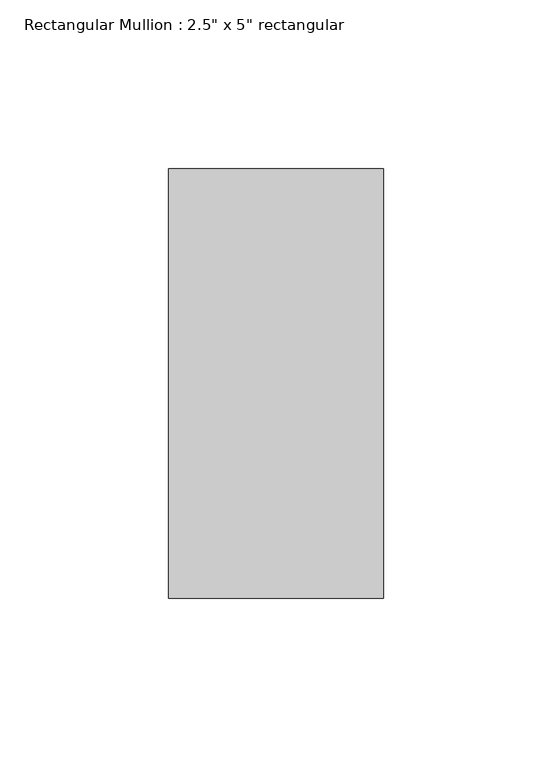
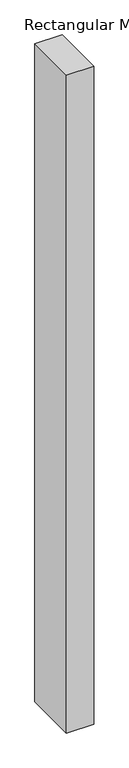
"""IFC4 building model written with IfcOpenShell, lengths in millimetres: member geometry."""

from ifc_helpers import new_model, si_unit, frame, origin, place, context, project, spatial, polyline, outline, extrude, source, transform, mapped, element, save


def member_25f01624(model_context):
    return source(origin(), model_context, "Body", "SweptSolid", [
        extrude(outline(polyline([(31.75, 63.5), (31.75, -63.5), (-31.75, -63.5), (-31.75, 63.5), (31.75, 63.5)])), frame((0.0, 0.0, -1616.3259354), z_axis=(0.0, 0.0, 1.0), x_axis=(1.0, 0.0, 0.0)), (0.0, 0.0, 1.0), 1616.3259354),
    ])


if __name__ == "__main__":
    model = new_model("IFC4")
    model_context = context("Model", 3, world=origin())
    ifc_project = project(units=[si_unit("LENGTHUNIT", "METRE", prefix="MILLI")], contexts=[model_context])
    site = spatial("IfcSite", under=ifc_project)
    building = spatial("IfcBuilding", under=site)
    placement = place(None, origin())
    member_shape = member_25f01624(model_context)
    element("IfcMember", 1, ObjectType="Rectangular Mullion : 2.5\" x 5\" rectangular", at=placement, inside=building, context=model_context, shape_type="MappedRepresentation", body=[
        mapped(member_shape, transform((0.0, 0.0, 0.0), x_axis=(1.0, 0.0, 0.0), y_axis=(0.0, 1.0, 0.0), z_axis=(0.0, 0.0, 1.0))),
    ])
    save(model, "model.ifc")

# Revit data of these elements
# Type "Rectangular Mullion : 2.5\" x 5\" rectangular"
#   built-in parameter 1007304 = 0.416667 (stored number, unit not read)
#   built-in parameter 1007301 = 0.104167 (stored number, unit not read)
#   built-in parameter 1007300 = 0.104167 (stored number, unit not read)
# Element 1 (IfcMember, "Rectangular Mullion : 2.5\" x 5\" rectangular")
#   Materials on its faces: "Aluminum"
# Materials
#   "Aluminum": class "Metal", colour RGB 247 247 247, transparency 0, Description = "Aluminum 6061", Cost = 0
